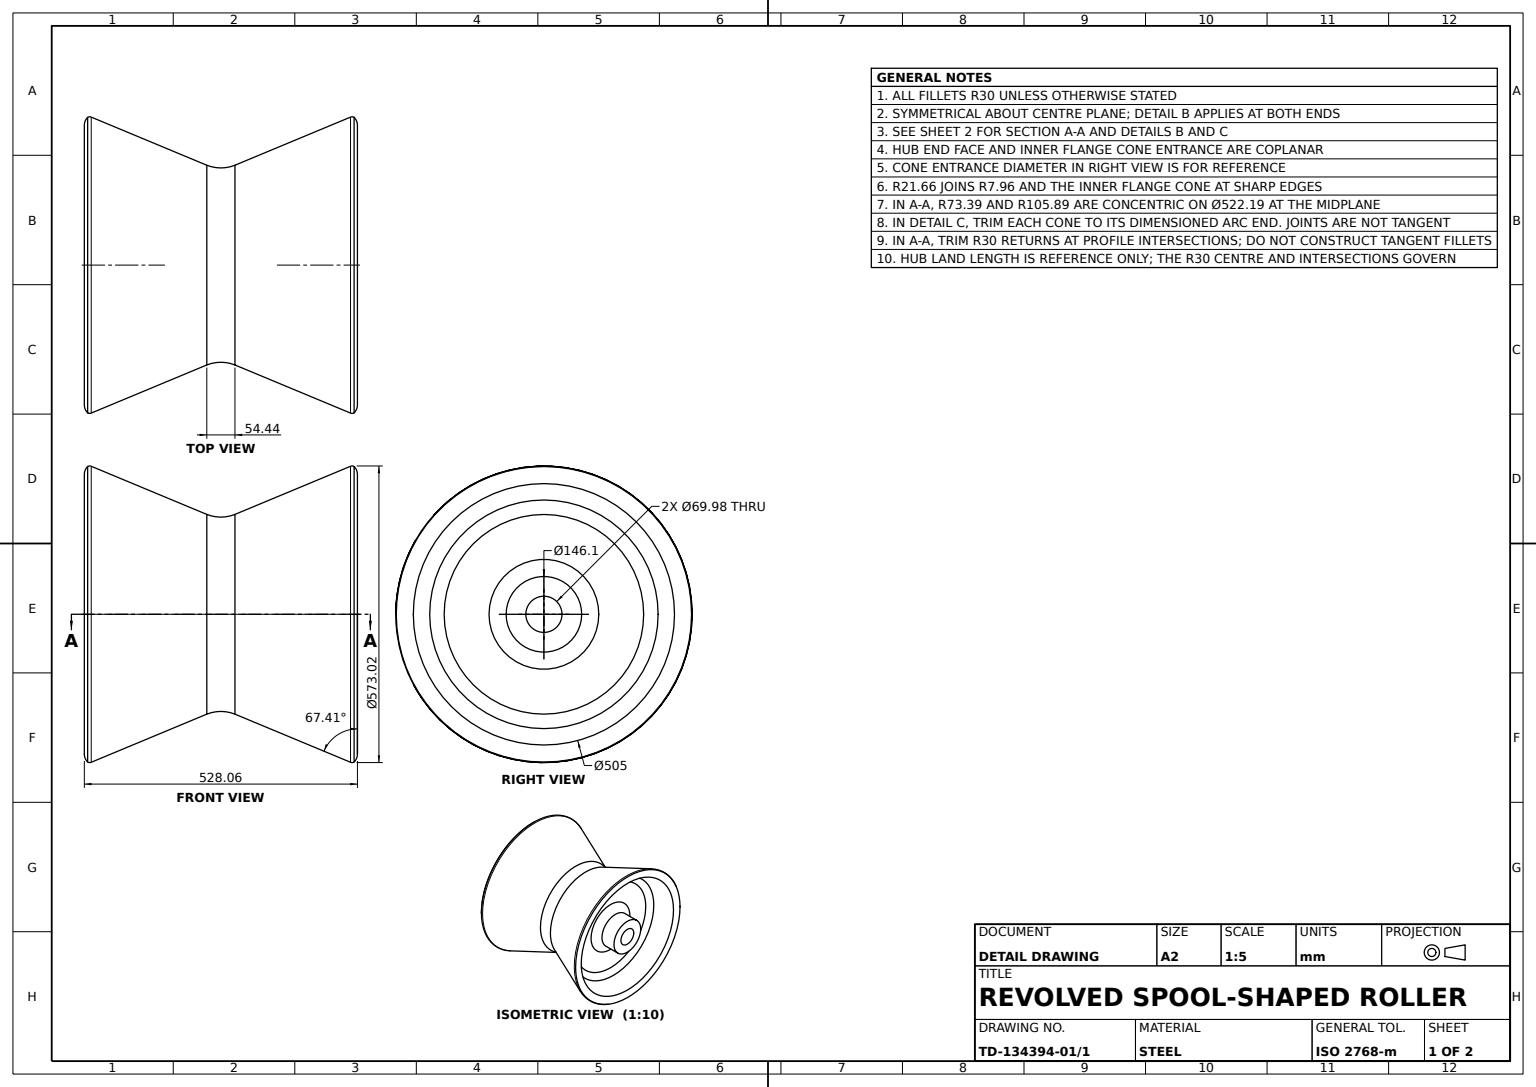
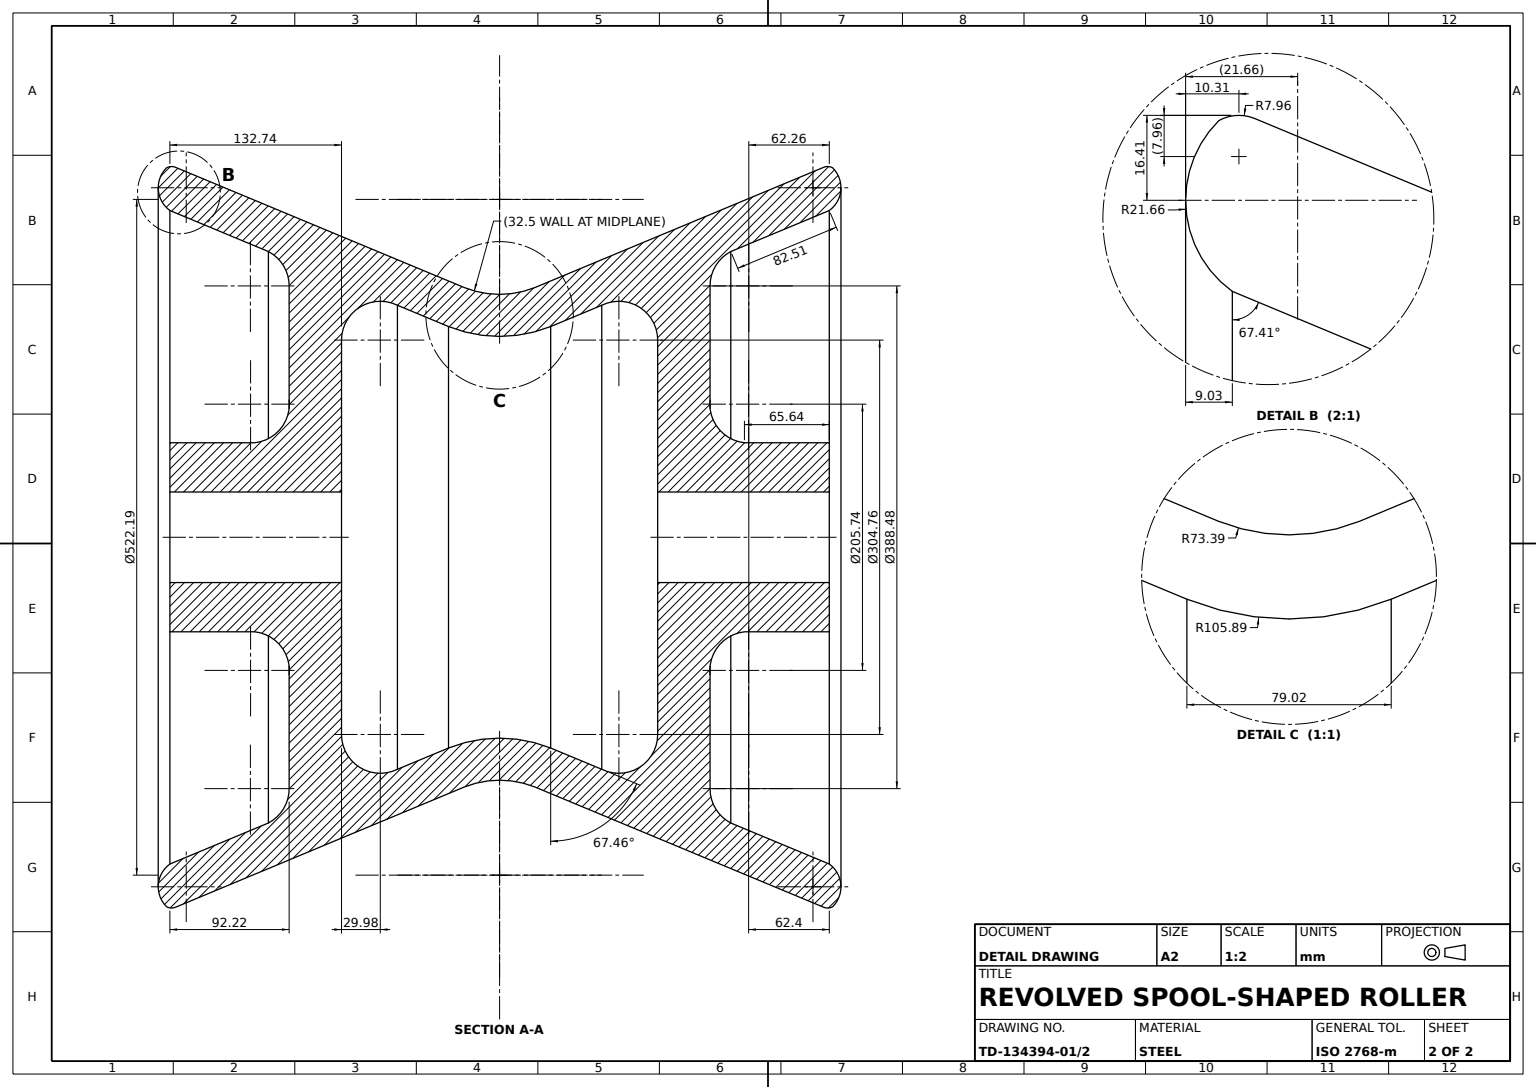
SolidWorks part; units mm, degrees
material "Plain Carbon Steel"
ref_plane "Front Plane" through (0, 0, 0) normal (0, 0, 1) x (1, 0, 0)
ref_plane "Top Plane" through (0, 0, 0) normal (0, 1, 0) x (1, 0, 0)
ref_plane "Right Plane" through (0, 0, 0) normal (1, 0, 0) x (0, 0, -1)
sketch "Cap Profile Sketch" plane through (0, 0, 0) normal (0, 0, 1) x (1, 0, 0)
  line L2 (288.5785, 67.4895) -> (288.5785, 183.9084)
  line L4 (-88.6836, 32.5) -> (421.3164, 32.5) construction
  line L5 (421.3164, 105.5482) -> (421.3164, 67.4895)
  line L6 (36.3164, 0) -> (36.3164, 32.5) construction
  line L8 (205.8263, 195.3554) -> (245.3363, 211.792)
  line L10 (421.3164, 67.4895) -> (288.5785, 67.4895)
  line L11 (193.5371, 225.4431) -> (417.0121, 318.4109)
  line L12 (-23.0423, 105.5482) -> (-88.6836, 105.5482)
  line L13 (193.3431, 225.3624) -> (232.0729, 241.4744) construction
  line L14 (205.8263, 195.3554) -> (248.8529, 213.2549)
  line L15 (329.0925, 228.1129) -> (329.0925, 138.6143)
  line L16 (453.8164, 99.9895) -> (321.0785, 99.9895) construction
  line L17 (321.0785, 99.9895) -> (321.0785, 183.4773) construction
  line L18 (453.8164, 0) -> (453.8164, 99.9895) construction
  line L19 (-88.6836, 0) -> (453.8164, 0) construction
  line L20 (345.1313, 253.3077) -> (421.3164, 285.0014)
  line L21 (355.675, 105.5482) -> (421.3164, 105.5482)
  line L22 (-12.4986, 253.3077) -> (-88.6836, 285.0014)
  line L23 (193.3431, 225.3624) -> (421.3164, 320.2015) construction
  line L24 (205.8263, 195.3554) -> (433.7996, 290.1945) construction
  line L25 (3.5402, 228.1129) -> (3.5402, 138.6143)
  line L26 (421.3164, 32.5) -> (421.3164, 67.4895) construction
  line L27 (126.8064, 195.3554) -> (83.7799, 213.2549)
  line L28 (139.0956, 225.4431) -> (-84.3793, 318.4109)
  line L29 (-88.6836, 67.4895) -> (44.0542, 67.4895)
  line L30 (126.8064, 195.3554) -> (87.2964, 211.792)
  line L31 (-88.6836, 105.5482) -> (-88.6836, 67.4895)
  line L32 (44.0542, 67.4895) -> (44.0542, 183.9084)
  line L33 (193.5371, 225.4431) -> (236.3697, 243.2619)
  arc A0 (245.3363, 211.792) -> (288.5785, 183.9084) centre (258.5943, 184.8805) cw
  arc A1 (126.8064, 195.3554) -> (205.8263, 195.3554) centre (166.3164, 293.5951) ccw
  arc A2 (193.3431, 225.3624) -> (193.3431, 225.3624) centre (193.3431, 225.3624) ccw
  arc A3 (205.8263, 195.3554) -> (205.8263, 195.3554) centre (205.8263, 195.3554) ccw
  arc A4 (232.0729, 241.4744) -> (321.0785, 183.4773) centre (258.5943, 184.8805) cw construction
  arc A5 (329.0925, 138.6143) -> (355.675, 105.5482) centre (358.9169, 135.3725) ccw
  arc A6 (329.0925, 225.3624) -> (345.1313, 253.3077) centre (359.061, 226.7377) cw
  arc A7 (423.926, 317.9971) -> (421.3164, 285.0014) centre (408.6854, 302.6014) cw
  arc A8 (417.0121, 318.4109) -> (423.926, 317.9971) centre (420.0408, 311.0476) cw
  arc A9 (138.9332, 225.5082) -> (193.5371, 225.4431) centre (166.3164, 293.5951) ccw
  arc A10 (-84.3793, 318.4109) -> (-91.2933, 317.9971) centre (-87.408, 311.0476) ccw
  arc A11 (-91.2933, 317.9971) -> (-88.6836, 285.0014) centre (-76.0527, 302.6014) ccw
  arc A12 (3.5402, 225.3624) -> (-12.4986, 253.3077) centre (-26.4283, 226.7377) ccw
  arc A13 (3.5402, 138.6143) -> (-23.0423, 105.5482) centre (-26.2841, 135.3725) cw
  arc A14 (87.2964, 211.792) -> (44.0542, 183.9084) centre (74.0384, 184.8805) ccw
  arc A15 (166.3164, 211.792) -> (205.8263, 195.3554) centre (191.038, 215.5124) ccw construction
  arc A16 (193.5371, 225.4431) -> (193.5371, 225.4431) centre (193.5371, 225.4431) ccw
  point P5 (288.5785, 0)
  point P6 (288.5785, 230)
  point P8 (36.3164, 230)
  dimension "D1" = 36.3164
  dimension "D2" = 32.5
  dimension "D14" = 30
  dimension "D15" = 21.6634
  dimension "D16" = 7.9618
  dimension "D17" = 105.887
  dimension "D25" = 73.387
  dimension "D3" = 421.3164
  dimension "D5" = 38.0586
  dimension "D4" = 67.4895
  dimension "D6" = 132.7378
  dimension "D7" = 116.4189
  dimension "D8" = 65.6413
  dimension "D9" = 89.4986
  dimension "D10" = 82.5145
  dimension "D11" = 242.0414
  dimension "D12" = 42.7925
  dimension "D13" = 46.6012
  dimension "D18" = 179.4532
  dimension "D19" = 92.2238
  dimension "D20" = 33.0662
  dimension "D21" = 86.7481
  dimension "D22" = 255
  dimension "D23" = 293.5951
  dimension "D24" = 79.0199
  dimension "D26" = 6.9495
  dimension "D27" = 3.0287
revolve "Cap Body Revolve 360" add sketch "Cap Profile Sketch" angle 360 about L4
